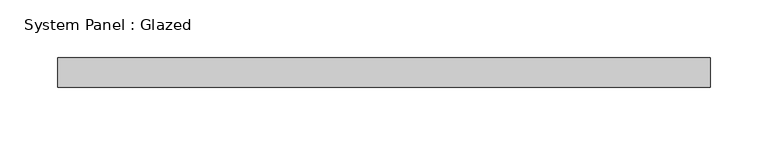
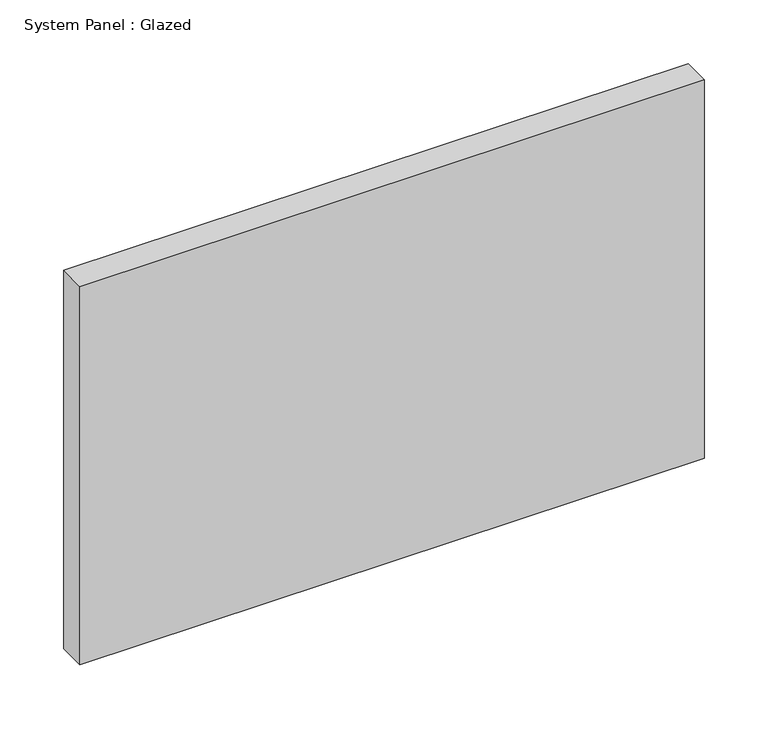
"""IFC4 building model written with IfcOpenShell, lengths in millimetres: plate geometry, System Panel : Glazed."""

from ifc_helpers import new_model, si_unit, origin, origin_with_axes, place, context, project, spatial, polyline, outline, extrude, source, transform, mapped, element, save


def system_panel_glazed_0dc12997(model_context):
    return source(origin(), model_context, "Body", "SweptSolid", [
        extrude(outline(polyline([(282.575, 19.05), (-282.575, 19.05), (-282.575, 44.45), (282.575, 44.45), (282.575, 19.05)])), origin_with_axes(), (0.0, 0.0, 1.0), 361.95),
    ])


if __name__ == "__main__":
    model = new_model("IFC4")
    model_context = context("Model", 3, world=origin())
    ifc_project = project(units=[si_unit("LENGTHUNIT", "METRE", prefix="MILLI")], contexts=[model_context])
    site = spatial("IfcSite", under=ifc_project)
    building = spatial("IfcBuilding", under=site)
    placement = place(None, origin())
    system_panel_glazed_shape = system_panel_glazed_0dc12997(model_context)
    element("IfcPlate", 1, ObjectType="System Panel : Glazed", at=placement, inside=building, context=model_context, shape_type="MappedRepresentation", body=[
        mapped(system_panel_glazed_shape, transform((0.0, 0.0, 0.0), x_axis=(1.0, 0.0, 0.0), y_axis=(0.0, 1.0, 0.0), z_axis=(0.0, 0.0, 1.0))),
    ])
    save(model, "model.ifc")

# Revit data of these elements
# Type "System Panel : Glazed"
#   Construction Type Id = "GSP4R"
#   Analytic Construction = "1/8 in Pilkington single glazing"
#   Visual Light Transmittance = 0.9
#   Solar Heat Gain Coefficient = 0.86
#   Heat Transfer Coefficient (U) = 1.18115 BTU/(h·ft²·°F)
#   Define Thermal Properties by = 1
# Element 1 (IfcPlate, "System Panel : Glazed")
#   Materials on its faces: "Glass"
# Materials
#   "Glass": class "Glass", colour RGB 0 128 192, transparency 0.75, Description = "Soda Lime Glass", Cost = 0
